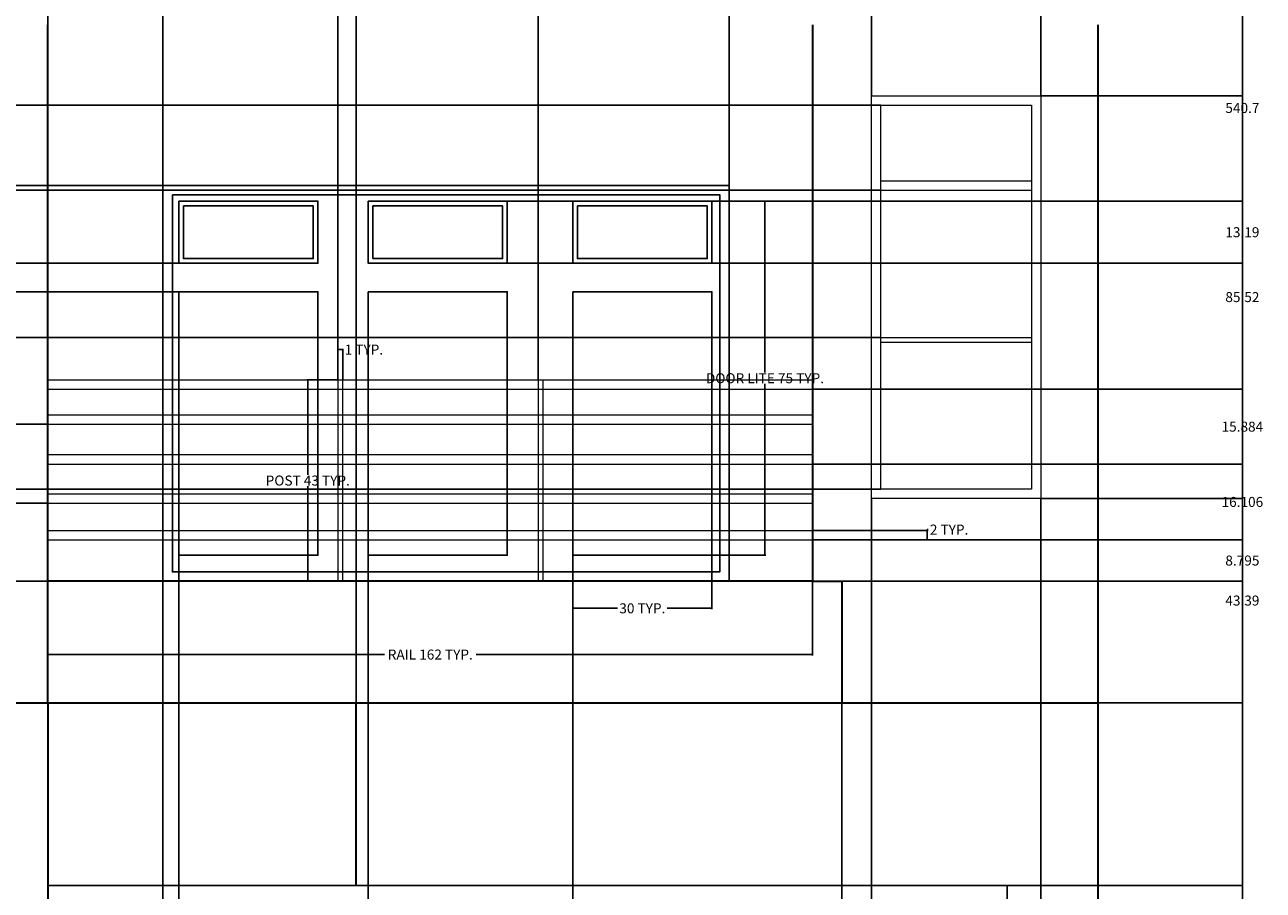
# Model space of a CAD drawing. Units: inches. Extents: x -113 to 379, y 13 to 689.
# Tile 3 of 5: x 116 to 379, y 221 to 405. Entities that reach past the tile are written whole.
import ezdxf

# ---------------------------------------------------------------- set-up
doc = ezdxf.new("R2010")
doc.units = ezdxf.units.IN
doc.header["$MEASUREMENT"] = 0
for name, color, linetype, lineweight in [('A-ANNO-DIMS', 2, 'Continuous', 18), ('A-DOOR', 3, 'Continuous', 25), ('A-FLOR', 7, 'Continuous', 30), ('A-FLOR-HRAL', 5, 'Continuous', 18), ('A-GLAZ', 4, 'Continuous', 18), ('A-WALL', 7, 'Continuous', 35)]:
    doc.layers.add(name, color=color, linetype=linetype, lineweight=lineweight)
doc.styles.get("Standard").update_dxf_attribs({"font": 'arial.ttf'})
doc.dimstyles.get("Standard").update_dxf_attribs({"dimtxt": 2.125, "dimasz": 0.18, "dimexe": 0.18, "dimexo": 0.0625, "dimgap": 0.09, "dimtad": 0, "dimtih": 1, "dimtoh": 1, "dimdec": 4, "dimzin": 0, "dimdsep": 46, "dimlunit": 4, "dimtxsty": 'Standard', "dimcen": 0.09, "dimadec": 0, "dimazin": 0, "dimtfac": 1, "dimtdec": 4, "dimtofl": 0, "dimtmove": 0, "dimatfit": 3, "dimfxl": 1, "dimtolj": 1, "dimtzin": 0, "dimarcsym": 0})

# ---------------------------------------------------------------- blocks, each defined once
blk = doc.blocks.new('BALCONY-DOOR-LITE')
for points in [[(0, 75.21), (29.55, 75.21), (29.55, 62.02), (0, 62.02)], [(1, 74.21), (28.55, 74.21), (28.55, 63.02), (1, 63.02)], [(0, 55.96), (29.55, 55.96), (29.55, 0), (0, 0)]]:
    blk.add_lwpolyline(points, close=True)
blk = doc.blocks.new('BALCONY-RAIL')
for p, q in [((0, 2), (162.45, 2)), ((0, 0), (162.45, 0))]:
    blk.add_line(p, q)
blk = doc.blocks.new('BALCONY-RAIL-POST')
for p, q in [((0, 42.78), (0, 0)), ((1, 42.78), (1, 0))]:
    blk.add_line(p, q)
blk = doc.blocks.new('*D13')
at = {"layer": 'A-ANNO-DIMS', "color": 0, "lineweight": -2, "transparency": 16777216}
for p, q in [((261.87, 367.18), (273.26, 367.18)), ((273.08, 367), (273.08, 330.77)), ((273.08, 292.16), (273.08, 328.39)), ((261.87, 291.98), (273.26, 291.98))]:
    blk.add_line(p, q, dxfattribs=at)
at = {"layer": 'A-ANNO-DIMS', "color": 0, "transparency": 16777216}
for points in [[(273.05, 367), (273.11, 367), (273.08, 367.18)], [(273.05, 292.16), (273.11, 292.16), (273.08, 291.98)]]:
    blk.add_solid(points, dxfattribs=at)
at = {"layer": 'Defpoints', "color": 0, "transparency": 16777216}
for p in [(261.8, 367.18), (273.08, 367.18), (261.8, 291.98)]:
    blk.add_point(p, dxfattribs=at)
at = {"layer": 'A-ANNO-DIMS', "color": 0, "transparency": 16777216, "insert": (273.08, 329.58), "char_height": 2.125, "attachment_point": 5}
blk.add_mtext('\\A1;DOOR LITE 75 TYP.', dxfattribs=at)
blk = doc.blocks.new('*D14')
at = {"layer": 'A-ANNO-DIMS', "color": 0, "lineweight": -2, "transparency": 16777216}
for p, q in [((232.25, 291.91), (232.25, 280.52)), ((261.8, 291.91), (261.8, 280.52)), ((232.43, 280.7), (241.77, 280.7)), ((261.62, 280.7), (252.29, 280.7))]:
    blk.add_line(p, q, dxfattribs=at)
at = {"layer": 'A-ANNO-DIMS', "color": 0, "transparency": 16777216}
for points in [[(232.43, 280.73), (232.43, 280.67), (232.25, 280.7)], [(261.62, 280.73), (261.62, 280.67), (261.8, 280.7)]]:
    blk.add_solid(points, dxfattribs=at)
at = {"layer": 'Defpoints', "color": 0, "transparency": 16777216}
for p in [(232.25, 291.98), (261.8, 291.98), (261.8, 280.7)]:
    blk.add_point(p, dxfattribs=at)
at = {"layer": 'A-ANNO-DIMS', "color": 0, "transparency": 16777216, "insert": (247.03, 280.7), "char_height": 2.125, "attachment_point": 5}
blk.add_mtext('\\A1;30 TYP.', dxfattribs=at)
blk = doc.blocks.new('*D15')
at = {"layer": 'A-ANNO-DIMS', "color": 0, "lineweight": -2, "transparency": 16777216}
for p, q in [((120.75, 295.18), (120.75, 270.7)), ((283.2, 295.18), (283.2, 270.7)), ((120.93, 270.88), (192.23, 270.88)), ((283.02, 270.88), (211.72, 270.88))]:
    blk.add_line(p, q, dxfattribs=at)
at = {"layer": 'A-ANNO-DIMS', "color": 0, "transparency": 16777216}
for points in [[(120.93, 270.91), (120.93, 270.85), (120.75, 270.88)], [(283.02, 270.91), (283.02, 270.85), (283.2, 270.88)]]:
    blk.add_solid(points, dxfattribs=at)
at = {"layer": 'Defpoints', "color": 0, "transparency": 16777216}
for p in [(120.75, 295.24), (283.2, 295.24), (283.2, 270.88)]:
    blk.add_point(p, dxfattribs=at)
at = {"layer": 'A-ANNO-DIMS', "color": 0, "transparency": 16777216, "insert": (201.98, 270.88), "char_height": 2.125, "attachment_point": 5}
blk.add_mtext('\\A1;RAIL 162 TYP.', dxfattribs=at)
blk = doc.blocks.new('*D16')
at = {"layer": 'A-ANNO-DIMS', "color": 0, "lineweight": -2, "transparency": 16777216}
for p, q in [((307.57, 297.24), (307.57, 297.42)), ((307.57, 297.42), (307.75, 297.42)), ((283.26, 297.24), (307.75, 297.24)), ((283.26, 295.24), (307.75, 295.24)), ((307.57, 295.42), (307.57, 297.06))]:
    blk.add_line(p, q, dxfattribs=at)
at = {"layer": 'A-ANNO-DIMS', "color": 0, "transparency": 16777216}
for points in [[(307.54, 297.06), (307.6, 297.06), (307.57, 297.24)], [(307.54, 295.42), (307.6, 295.42), (307.57, 295.24)]]:
    blk.add_solid(points, dxfattribs=at)
at = {"layer": 'Defpoints', "color": 0, "transparency": 16777216}
for p in [(283.2, 297.24), (283.2, 295.24), (307.57, 297.24)]:
    blk.add_point(p, dxfattribs=at)
at = {"layer": 'A-ANNO-DIMS', "color": 0, "transparency": 16777216, "insert": (312.2, 297.42), "char_height": 2.125, "attachment_point": 5}
blk.add_mtext('\\A1;2 TYP.', dxfattribs=at)
blk = doc.blocks.new('*D17')
at = {"layer": 'A-ANNO-DIMS', "color": 0, "lineweight": -2, "transparency": 16777216}
for p, q in [((182.31, 329.23), (175.77, 329.23)), ((175.95, 329.05), (175.95, 309.03)), ((175.95, 286.63), (175.95, 306.65)), ((182.31, 286.45), (175.77, 286.45))]:
    blk.add_line(p, q, dxfattribs=at)
at = {"layer": 'A-ANNO-DIMS', "color": 0, "transparency": 16777216}
for points in [[(175.92, 329.05), (175.98, 329.05), (175.95, 329.23)], [(175.92, 286.63), (175.98, 286.63), (175.95, 286.45)]]:
    blk.add_solid(points, dxfattribs=at)
at = {"layer": 'Defpoints', "color": 0, "transparency": 16777216}
for p in [(175.95, 329.23), (182.37, 329.23), (182.37, 286.45)]:
    blk.add_point(p, dxfattribs=at)
at = {"layer": 'A-ANNO-DIMS', "color": 0, "transparency": 16777216, "insert": (175.95, 307.84), "char_height": 2.125, "attachment_point": 5}
blk.add_mtext('\\A1;POST 43 TYP.', dxfattribs=at)
blk = doc.blocks.new('*D18')
at = {"layer": 'A-ANNO-DIMS', "color": 0, "lineweight": -2, "transparency": 16777216}
for p, q in [((182.37, 329.3), (182.37, 335.83)), ((182.55, 335.65), (183.19, 335.65)), ((183.37, 329.3), (183.37, 335.83)), ((183.37, 335.65), (183.55, 335.65))]:
    blk.add_line(p, q, dxfattribs=at)
at = {"layer": 'A-ANNO-DIMS', "color": 0, "transparency": 16777216}
for points in [[(182.55, 335.68), (182.55, 335.62), (182.37, 335.65)], [(183.19, 335.68), (183.19, 335.62), (183.37, 335.65)]]:
    blk.add_solid(points, dxfattribs=at)
at = {"layer": 'Defpoints', "color": 0, "transparency": 16777216}
for p in [(183.37, 335.65), (182.37, 329.23), (183.37, 329.23)]:
    blk.add_point(p, dxfattribs=at)
at = {"layer": 'A-ANNO-DIMS', "color": 0, "transparency": 16777216, "insert": (187.88, 335.65), "char_height": 2.125, "attachment_point": 5}
blk.add_mtext('\\A1;1 TYP.', dxfattribs=at)
blk = doc.blocks.new('*D20')
at = {"layer": 'A-ANNO-DIMS', "color": 0, "lineweight": -2, "transparency": 16777216}
for p, q in [((232.74, 657.3), (374.68, 657.3)), ((374.5, 657.12), (374.5, 388.15)), ((374.5, 116.83), (374.5, 385.8)), ((343.93, 116.65), (374.68, 116.65))]:
    blk.add_line(p, q, dxfattribs=at)
at = {"layer": 'A-ANNO-DIMS', "color": 0, "transparency": 16777216}
for points in [[(374.47, 657.12), (374.53, 657.12), (374.5, 657.3)], [(374.47, 116.83), (374.53, 116.83), (374.5, 116.65)]]:
    blk.add_solid(points, dxfattribs=at)
at = {"layer": 'Defpoints', "color": 0, "transparency": 16777216}
for p in [(232.68, 657.3), (374.5, 657.3), (343.87, 116.65)]:
    blk.add_point(p, dxfattribs=at)
at = {"layer": 'A-ANNO-DIMS', "color": 0, "transparency": 16777216, "insert": (374.5, 386.98), "char_height": 2.125, "attachment_point": 5}
blk.add_mtext('\\A1;540.7', dxfattribs=at)
blk = doc.blocks.new('*D33')
at = {"layer": 'A-ANNO-DIMS', "color": 0, "lineweight": -2, "transparency": 16777216}
for p, q in [((120.75, 221.89), (120.75, 688.12)), ((120.93, 687.94), (149.81, 687.94)), ((186.04, 687.94), (157.17, 687.94)), ((186.22, 221.89), (186.22, 688.12))]:
    blk.add_line(p, q, dxfattribs=at)
at = {"layer": 'A-ANNO-DIMS', "color": 0, "transparency": 16777216}
for points in [[(120.93, 687.97), (120.93, 687.91), (120.75, 687.94)], [(186.04, 687.97), (186.04, 687.91), (186.22, 687.94)]]:
    blk.add_solid(points, dxfattribs=at)
at = {"layer": 'Defpoints', "color": 0, "transparency": 16777216}
for p in [(186.22, 687.94), (120.75, 221.82), (186.22, 221.82)]:
    blk.add_point(p, dxfattribs=at)
at = {"layer": 'A-ANNO-DIMS', "color": 0, "transparency": 16777216, "insert": (153.49, 687.94), "char_height": 2.125, "attachment_point": 5}
blk.add_mtext('\\A1;65.47', dxfattribs=at)
blk = doc.blocks.new('*D35')
at = {"layer": 'A-ANNO-DIMS', "color": 0, "lineweight": -2, "transparency": 16777216}
for p, q in [((324.57, 221.82), (374.68, 221.82)), ((374.5, 221.64), (374.5, 170.41)), ((374.5, 116.83), (374.5, 168.06)), ((324.57, 116.65), (374.68, 116.65))]:
    blk.add_line(p, q, dxfattribs=at)
at = {"layer": 'A-ANNO-DIMS', "color": 0, "transparency": 16777216}
for points in [[(374.47, 221.64), (374.53, 221.64), (374.5, 221.82)], [(374.47, 116.83), (374.53, 116.83), (374.5, 116.65)]]:
    blk.add_solid(points, dxfattribs=at)
at = {"layer": 'Defpoints', "color": 0, "transparency": 16777216}
for p in [(324.51, 221.82), (374.5, 221.82), (324.51, 116.65)]:
    blk.add_point(p, dxfattribs=at)
at = {"layer": 'A-ANNO-DIMS', "color": 0, "transparency": 16777216, "insert": (374.5, 169.24), "char_height": 2.125, "attachment_point": 5}
blk.add_mtext('\\A1;105.17', dxfattribs=at)
blk = doc.blocks.new('*D38')
at = {"layer": 'A-ANNO-DIMS', "color": 0, "lineweight": -2, "transparency": 16777216}
for p, q in [((289.33, 286.45), (-108.66, 286.45)), ((-108.48, 286.27), (-108.48, 274.73)), ((-108.48, 260.83), (-108.48, 272.38)), ((289.33, 260.65), (-108.66, 260.65))]:
    blk.add_line(p, q, dxfattribs=at)
at = {"layer": 'A-ANNO-DIMS', "color": 0, "transparency": 16777216}
for points in [[(-108.51, 286.27), (-108.45, 286.27), (-108.48, 286.45)], [(-108.51, 260.83), (-108.45, 260.83), (-108.48, 260.65)]]:
    blk.add_solid(points, dxfattribs=at)
at = {"layer": 'Defpoints', "color": 0, "transparency": 16777216}
for p in [(-108.48, 286.45), (289.4, 286.45), (289.4, 260.65)]:
    blk.add_point(p, dxfattribs=at)
at = {"layer": 'A-ANNO-DIMS', "color": 0, "transparency": 16777216, "insert": (-108.48, 273.55), "char_height": 2.125, "attachment_point": 5}
blk.add_mtext('\\A1;25.8', dxfattribs=at)
blk = doc.blocks.new('*D39')
at = {"layer": 'A-ANNO-DIMS', "color": 0, "lineweight": -2, "transparency": 16777216}
for p, q in [((145.2, 370.61), (145.2, 688.12)), ((145.38, 687.94), (201.77, 687.94)), ((265.31, 687.94), (208.92, 687.94)), ((265.49, 370.61), (265.49, 688.12))]:
    blk.add_line(p, q, dxfattribs=at)
at = {"layer": 'A-ANNO-DIMS', "color": 0, "transparency": 16777216}
for points in [[(145.38, 687.97), (145.38, 687.91), (145.2, 687.94)], [(265.31, 687.97), (265.31, 687.91), (265.49, 687.94)]]:
    blk.add_solid(points, dxfattribs=at)
at = {"layer": 'Defpoints', "color": 0, "transparency": 16777216}
for p in [(265.49, 687.94), (145.2, 370.54), (265.49, 370.54)]:
    blk.add_point(p, dxfattribs=at)
at = {"layer": 'A-ANNO-DIMS', "color": 0, "transparency": 16777216, "insert": (205.34, 687.94), "char_height": 2.125, "attachment_point": 5}
blk.add_mtext('\\A1;120.3', dxfattribs=at)
blk = doc.blocks.new('*D40')
at = {"layer": 'A-ANNO-DIMS', "color": 0, "lineweight": -2, "transparency": 16777216}
for p, q in [((145.14, 370.54), (-108.66, 370.54)), ((-108.48, 370.36), (-108.48, 329.67)), ((-108.48, 286.63), (-108.48, 327.32)), ((145.14, 286.45), (-108.66, 286.45))]:
    blk.add_line(p, q, dxfattribs=at)
at = {"layer": 'A-ANNO-DIMS', "color": 0, "transparency": 16777216}
for points in [[(-108.51, 370.36), (-108.45, 370.36), (-108.48, 370.54)], [(-108.51, 286.63), (-108.45, 286.63), (-108.48, 286.45)]]:
    blk.add_solid(points, dxfattribs=at)
at = {"layer": 'Defpoints', "color": 0, "transparency": 16777216}
for p in [(-108.48, 370.54), (145.2, 370.54), (145.2, 286.45)]:
    blk.add_point(p, dxfattribs=at)
at = {"layer": 'A-ANNO-DIMS', "color": 0, "transparency": 16777216, "insert": (-108.48, 328.5), "char_height": 2.125, "attachment_point": 5}
blk.add_mtext('\\A1;84.1', dxfattribs=at)
blk = doc.blocks.new('*D41')
at = {"layer": 'A-ANNO-DIMS', "color": 0, "lineweight": -2, "transparency": 16777216}
for p, q in [((120.75, 286.39), (120.75, 13.95)), ((145.2, 286.39), (145.2, 13.95)), ((120.93, 14.13), (128.45, 14.13)), ((145.02, 14.13), (137.5, 14.13))]:
    blk.add_line(p, q, dxfattribs=at)
at = {"layer": 'A-ANNO-DIMS', "color": 0, "transparency": 16777216}
for points in [[(120.93, 14.16), (120.93, 14.1), (120.75, 14.13)], [(145.02, 14.16), (145.02, 14.1), (145.2, 14.13)]]:
    blk.add_solid(points, dxfattribs=at)
at = {"layer": 'Defpoints', "color": 0, "transparency": 16777216}
for p in [(120.75, 286.45), (145.2, 286.45), (145.2, 14.13)]:
    blk.add_point(p, dxfattribs=at)
at = {"layer": 'A-ANNO-DIMS', "color": 0, "transparency": 16777216, "insert": (132.98, 14.13), "char_height": 2.125, "attachment_point": 5}
blk.add_mtext('\\A1;24.445', dxfattribs=at)
blk = doc.blocks.new('*D42')
at = {"layer": 'A-ANNO-DIMS', "color": 0, "lineweight": -2, "transparency": 16777216}
for p, q in [((295.73, 389.63), (295.73, 688.12)), ((295.91, 687.94), (309.2, 687.94)), ((331.5, 687.94), (318.21, 687.94)), ((331.68, 389.63), (331.68, 688.12))]:
    blk.add_line(p, q, dxfattribs=at)
at = {"layer": 'A-ANNO-DIMS', "color": 0, "transparency": 16777216}
for points in [[(295.91, 687.97), (295.91, 687.91), (295.73, 687.94)], [(331.5, 687.97), (331.5, 687.91), (331.68, 687.94)]]:
    blk.add_solid(points, dxfattribs=at)
at = {"layer": 'Defpoints', "color": 0, "transparency": 16777216}
for p in [(331.68, 687.94), (295.73, 389.57), (331.68, 389.57)]:
    blk.add_point(p, dxfattribs=at)
at = {"layer": 'A-ANNO-DIMS', "color": 0, "transparency": 16777216, "insert": (313.71, 687.94), "char_height": 2.125, "attachment_point": 5}
blk.add_mtext('\\A1;35.955', dxfattribs=at)
blk = doc.blocks.new('*D43')
at = {"layer": 'A-ANNO-DIMS', "color": 0, "lineweight": -2, "transparency": 16777216}
for p, q in [((331.75, 389.57), (374.68, 389.57)), ((374.5, 389.39), (374.5, 347.98)), ((374.5, 304.22), (374.5, 345.63)), ((331.75, 304.04), (374.68, 304.04))]:
    blk.add_line(p, q, dxfattribs=at)
at = {"layer": 'A-ANNO-DIMS', "color": 0, "transparency": 16777216}
for points in [[(374.47, 389.39), (374.53, 389.39), (374.5, 389.57)], [(374.47, 304.22), (374.53, 304.22), (374.5, 304.04)]]:
    blk.add_solid(points, dxfattribs=at)
at = {"layer": 'Defpoints', "color": 0, "transparency": 16777216}
for p in [(331.68, 389.57), (374.5, 389.57), (331.68, 304.04)]:
    blk.add_point(p, dxfattribs=at)
at = {"layer": 'A-ANNO-DIMS', "color": 0, "transparency": 16777216, "insert": (374.5, 346.81), "char_height": 2.125, "attachment_point": 5}
blk.add_mtext('\\A1;85.52', dxfattribs=at)
blk = doc.blocks.new('*D44')
at = {"layer": 'A-ANNO-DIMS', "color": 0, "lineweight": -2, "transparency": 16777216}
for p, q in [((331.68, 303.98), (331.68, 13.95)), ((343.87, 260.59), (343.87, 13.95)), ((331.86, 14.13), (333.38, 14.13)), ((343.69, 14.13), (342.18, 14.13))]:
    blk.add_line(p, q, dxfattribs=at)
at = {"layer": 'A-ANNO-DIMS', "color": 0, "transparency": 16777216}
for points in [[(331.86, 14.16), (331.86, 14.1), (331.68, 14.13)], [(343.69, 14.16), (343.69, 14.1), (343.87, 14.13)]]:
    blk.add_solid(points, dxfattribs=at)
at = {"layer": 'Defpoints', "color": 0, "transparency": 16777216}
for p in [(331.68, 304.04), (343.87, 260.65), (343.87, 14.13)]:
    blk.add_point(p, dxfattribs=at)
at = {"layer": 'A-ANNO-DIMS', "color": 0, "transparency": 16777216, "insert": (337.78, 14.13), "char_height": 2.125, "attachment_point": 5}
blk.add_mtext('\\A1;12.186', dxfattribs=at)
blk = doc.blocks.new('*D45')
at = {"layer": 'A-ANNO-DIMS', "color": 0, "lineweight": -2, "transparency": 16777216}
for p, q in [((331.75, 304.04), (374.68, 304.04)), ((374.5, 303.86), (374.5, 283.52)), ((374.5, 260.83), (374.5, 281.17)), ((343.93, 260.65), (374.68, 260.65))]:
    blk.add_line(p, q, dxfattribs=at)
at = {"layer": 'A-ANNO-DIMS', "color": 0, "transparency": 16777216}
for points in [[(374.47, 303.86), (374.53, 303.86), (374.5, 304.04)], [(374.47, 260.83), (374.53, 260.83), (374.5, 260.65)]]:
    blk.add_solid(points, dxfattribs=at)
at = {"layer": 'Defpoints', "color": 0, "transparency": 16777216}
for p in [(331.68, 304.04), (343.87, 260.65), (374.5, 260.65)]:
    blk.add_point(p, dxfattribs=at)
at = {"layer": 'A-ANNO-DIMS', "color": 0, "transparency": 16777216, "insert": (374.5, 282.35), "char_height": 2.125, "attachment_point": 5}
blk.add_mtext('\\A1;43.39', dxfattribs=at)
blk = doc.blocks.new('*D46')
at = {"layer": 'A-ANNO-DIMS', "color": 0, "lineweight": -2, "transparency": 16777216}
for p, q in [((295.73, 303.98), (295.73, 13.95)), ((289.4, 260.59), (289.4, 13.95)), ((289.58, 14.13), (295.55, 14.13)), ((295.73, 14.13), (295.91, 14.13))]:
    blk.add_line(p, q, dxfattribs=at)
at = {"layer": 'A-ANNO-DIMS', "color": 0, "transparency": 16777216}
for points in [[(289.58, 14.16), (289.58, 14.1), (289.4, 14.13)], [(295.55, 14.16), (295.55, 14.1), (295.73, 14.13)]]:
    blk.add_solid(points, dxfattribs=at)
at = {"layer": 'Defpoints', "color": 0, "transparency": 16777216}
for p in [(295.73, 304.04), (289.4, 260.65), (295.73, 14.13)]:
    blk.add_point(p, dxfattribs=at)
at = {"layer": 'A-ANNO-DIMS', "color": 0, "transparency": 16777216, "insert": (299.58, 14.13), "char_height": 2.125, "attachment_point": 5}
blk.add_mtext('\\A1;6.332', dxfattribs=at)
blk = doc.blocks.new('*D56')
at = {"layer": 'A-ANNO-DIMS', "color": 0, "lineweight": -2, "transparency": 16777216}
for p, q in [((148.55, 291.91), (148.55, 13.95)), ((188.79, 291.91), (188.79, 13.95)), ((148.73, 14.13), (164.96, 14.13)), ((188.61, 14.13), (172.39, 14.13))]:
    blk.add_line(p, q, dxfattribs=at)
at = {"layer": 'A-ANNO-DIMS', "color": 0, "transparency": 16777216}
for points in [[(148.73, 14.16), (148.73, 14.1), (148.55, 14.13)], [(188.61, 14.16), (188.61, 14.1), (188.79, 14.13)]]:
    blk.add_solid(points, dxfattribs=at)
at = {"layer": 'Defpoints', "color": 0, "transparency": 16777216}
for p in [(148.55, 291.98), (188.79, 291.98), (188.79, 14.13)]:
    blk.add_point(p, dxfattribs=at)
at = {"layer": 'A-ANNO-DIMS', "color": 0, "transparency": 16777216, "insert": (168.67, 14.13), "char_height": 2.125, "attachment_point": 5}
blk.add_mtext('\\A1;40.24', dxfattribs=at)
blk = doc.blocks.new('*D57')
at = {"layer": 'A-ANNO-DIMS', "color": 0, "lineweight": -2, "transparency": 16777216}
for p, q in [((188.79, 291.91), (188.79, 13.95)), ((232.25, 291.91), (232.25, 13.95)), ((188.97, 14.13), (206.81, 14.13)), ((232.07, 14.13), (214.24, 14.13))]:
    blk.add_line(p, q, dxfattribs=at)
at = {"layer": 'A-ANNO-DIMS', "color": 0, "transparency": 16777216}
for points in [[(188.97, 14.16), (188.97, 14.1), (188.79, 14.13)], [(232.07, 14.16), (232.07, 14.1), (232.25, 14.13)]]:
    blk.add_solid(points, dxfattribs=at)
at = {"layer": 'Defpoints', "color": 0, "transparency": 16777216}
for p in [(188.79, 291.98), (232.25, 291.98), (232.25, 14.13)]:
    blk.add_point(p, dxfattribs=at)
at = {"layer": 'A-ANNO-DIMS', "color": 0, "transparency": 16777216, "insert": (210.52, 14.13), "char_height": 2.125, "attachment_point": 5}
blk.add_mtext('\\A1;43.46', dxfattribs=at)
blk = doc.blocks.new('*D58')
at = {"layer": 'A-ANNO-DIMS', "color": 0, "lineweight": -2, "transparency": 16777216}
for p, q in [((182.37, 329.3), (182.37, 688.12)), ((182.55, 687.94), (199.91, 687.94)), ((224.72, 687.94), (207.35, 687.94)), ((224.9, 329.3), (224.9, 688.12))]:
    blk.add_line(p, q, dxfattribs=at)
at = {"layer": 'A-ANNO-DIMS', "color": 0, "transparency": 16777216}
for points in [[(182.55, 687.97), (182.55, 687.91), (182.37, 687.94)], [(224.72, 687.97), (224.72, 687.91), (224.9, 687.94)]]:
    blk.add_solid(points, dxfattribs=at)
at = {"layer": 'Defpoints', "color": 0, "transparency": 16777216}
for p in [(224.9, 687.94), (182.37, 329.23), (224.9, 329.23)]:
    blk.add_point(p, dxfattribs=at)
at = {"layer": 'A-ANNO-DIMS', "color": 0, "transparency": 16777216, "insert": (203.63, 687.94), "char_height": 2.125, "attachment_point": 5}
blk.add_mtext('\\A1;42.53', dxfattribs=at)
blk = doc.blocks.new('*D59')
at = {"layer": 'A-ANNO-DIMS', "color": 0, "lineweight": -2, "transparency": 16777216}
for p, q in [((120.75, 329.3), (120.75, 688.12)), ((120.93, 687.94), (148.08, 687.94)), ((182.19, 687.94), (155.04, 687.94)), ((182.37, 329.3), (182.37, 688.12))]:
    blk.add_line(p, q, dxfattribs=at)
at = {"layer": 'A-ANNO-DIMS', "color": 0, "transparency": 16777216}
for points in [[(120.93, 687.97), (120.93, 687.91), (120.75, 687.94)], [(182.19, 687.97), (182.19, 687.91), (182.37, 687.94)]]:
    blk.add_solid(points, dxfattribs=at)
at = {"layer": 'Defpoints', "color": 0, "transparency": 16777216}
for p in [(182.37, 687.94), (120.75, 329.23), (182.37, 329.23)]:
    blk.add_point(p, dxfattribs=at)
at = {"layer": 'A-ANNO-DIMS', "color": 0, "transparency": 16777216, "insert": (151.56, 687.94), "char_height": 2.125, "attachment_point": 5}
blk.add_mtext('\\A1;61.61', dxfattribs=at)
blk = doc.blocks.new('*D60')
at = {"layer": 'A-ANNO-DIMS', "color": 0, "lineweight": -2, "transparency": 16777216}
for p, q in [((120.69, 303.02), (-108.66, 303.02)), ((-108.48, 302.84), (-108.48, 295.91)), ((-108.48, 286.63), (-108.48, 293.56)), ((120.69, 286.45), (-108.66, 286.45))]:
    blk.add_line(p, q, dxfattribs=at)
at = {"layer": 'A-ANNO-DIMS', "color": 0, "transparency": 16777216}
for points in [[(-108.51, 302.84), (-108.45, 302.84), (-108.48, 303.02)], [(-108.51, 286.63), (-108.45, 286.63), (-108.48, 286.45)]]:
    blk.add_solid(points, dxfattribs=at)
at = {"layer": 'Defpoints', "color": 0, "transparency": 16777216}
for p in [(-108.48, 303.02), (120.75, 303.02), (120.75, 286.45)]:
    blk.add_point(p, dxfattribs=at)
at = {"layer": 'A-ANNO-DIMS', "color": 0, "transparency": 16777216, "insert": (-108.48, 294.73), "char_height": 2.125, "attachment_point": 5}
blk.add_mtext('\\A1;16.566', dxfattribs=at)
blk = doc.blocks.new('*D61')
at = {"layer": 'A-ANNO-DIMS', "color": 0, "lineweight": -2, "transparency": 16777216}
for p, q in [((120.69, 319.8), (-108.66, 319.8)), ((-108.48, 319.62), (-108.48, 312.58)), ((-108.48, 303.2), (-108.48, 310.23)), ((120.69, 303.02), (-108.66, 303.02))]:
    blk.add_line(p, q, dxfattribs=at)
at = {"layer": 'A-ANNO-DIMS', "color": 0, "transparency": 16777216}
for points in [[(-108.51, 319.62), (-108.45, 319.62), (-108.48, 319.8)], [(-108.51, 303.2), (-108.45, 303.2), (-108.48, 303.02)]]:
    blk.add_solid(points, dxfattribs=at)
at = {"layer": 'Defpoints', "color": 0, "transparency": 16777216}
for p in [(-108.48, 319.8), (120.75, 319.8), (120.75, 303.02)]:
    blk.add_point(p, dxfattribs=at)
at = {"layer": 'A-ANNO-DIMS', "color": 0, "transparency": 16777216, "insert": (-108.48, 311.41), "char_height": 2.125, "attachment_point": 5}
blk.add_mtext('\\A1;16.788', dxfattribs=at)
blk = doc.blocks.new('*D62')
at = {"layer": 'A-ANNO-DIMS', "color": 0, "lineweight": -2, "transparency": 16777216}
for p, q in [((283.26, 295.24), (374.68, 295.24)), ((374.5, 295.06), (374.5, 292.02)), ((374.5, 286.63), (374.5, 289.67)), ((283.26, 286.45), (374.68, 286.45))]:
    blk.add_line(p, q, dxfattribs=at)
at = {"layer": 'A-ANNO-DIMS', "color": 0, "transparency": 16777216}
for points in [[(374.47, 295.06), (374.53, 295.06), (374.5, 295.24)], [(374.47, 286.63), (374.53, 286.63), (374.5, 286.45)]]:
    blk.add_solid(points, dxfattribs=at)
at = {"layer": 'Defpoints', "color": 0, "transparency": 16777216}
for p in [(283.2, 295.24), (374.5, 295.24), (283.2, 286.45)]:
    blk.add_point(p, dxfattribs=at)
at = {"layer": 'A-ANNO-DIMS', "color": 0, "transparency": 16777216, "insert": (374.5, 290.85), "char_height": 2.125, "attachment_point": 5}
blk.add_mtext('\\A1;8.795', dxfattribs=at)
blk = doc.blocks.new('*D63')
at = {"layer": 'A-ANNO-DIMS', "color": 0, "lineweight": -2, "transparency": 16777216}
for p, q in [((283.26, 311.35), (374.68, 311.35)), ((374.5, 311.17), (374.5, 304.47)), ((374.5, 295.42), (374.5, 302.12)), ((283.26, 295.24), (374.68, 295.24))]:
    blk.add_line(p, q, dxfattribs=at)
at = {"layer": 'A-ANNO-DIMS', "color": 0, "transparency": 16777216}
for points in [[(374.47, 311.17), (374.53, 311.17), (374.5, 311.35)], [(374.47, 295.42), (374.53, 295.42), (374.5, 295.24)]]:
    blk.add_solid(points, dxfattribs=at)
at = {"layer": 'Defpoints', "color": 0, "transparency": 16777216}
for p in [(283.2, 311.35), (374.5, 311.35), (283.2, 295.24)]:
    blk.add_point(p, dxfattribs=at)
at = {"layer": 'A-ANNO-DIMS', "color": 0, "transparency": 16777216, "insert": (374.5, 303.3), "char_height": 2.125, "attachment_point": 5}
blk.add_mtext('\\A1;16.106', dxfattribs=at)
blk = doc.blocks.new('*D64')
at = {"layer": 'A-ANNO-DIMS', "color": 0, "lineweight": -2, "transparency": 16777216}
for p, q in [((283.26, 327.23), (374.68, 327.23)), ((374.5, 327.05), (374.5, 320.47)), ((374.5, 311.53), (374.5, 318.12)), ((283.26, 311.35), (374.68, 311.35))]:
    blk.add_line(p, q, dxfattribs=at)
at = {"layer": 'A-ANNO-DIMS', "color": 0, "transparency": 16777216}
for points in [[(374.47, 327.05), (374.53, 327.05), (374.5, 327.23)], [(374.47, 311.53), (374.53, 311.53), (374.5, 311.35)]]:
    blk.add_solid(points, dxfattribs=at)
at = {"layer": 'Defpoints', "color": 0, "transparency": 16777216}
for p in [(283.2, 327.23), (374.5, 327.23), (283.2, 311.35)]:
    blk.add_point(p, dxfattribs=at)
at = {"layer": 'A-ANNO-DIMS', "color": 0, "transparency": 16777216, "insert": (374.5, 319.29), "char_height": 2.125, "attachment_point": 5}
blk.add_mtext('\\A1;15.884', dxfattribs=at)
blk = doc.blocks.new('*D65')
at = {"layer": 'A-ANNO-DIMS', "color": 0, "lineweight": -2, "transparency": 16777216}
for p, q in [((297.67, 338.26), (-108.66, 338.26)), ((-108.48, 338.08), (-108.48, 323.33)), ((-108.48, 306.22), (-108.48, 320.98)), ((297.67, 306.04), (-108.66, 306.04))]:
    blk.add_line(p, q, dxfattribs=at)
at = {"layer": 'A-ANNO-DIMS', "color": 0, "transparency": 16777216}
for points in [[(-108.51, 338.08), (-108.45, 338.08), (-108.48, 338.26)], [(-108.51, 306.22), (-108.45, 306.22), (-108.48, 306.04)]]:
    blk.add_solid(points, dxfattribs=at)
at = {"layer": 'Defpoints', "color": 0, "transparency": 16777216}
for p in [(-108.48, 338.26), (297.73, 338.26), (297.73, 306.04)]:
    blk.add_point(p, dxfattribs=at)
at = {"layer": 'A-ANNO-DIMS', "color": 0, "transparency": 16777216, "insert": (-108.48, 322.15), "char_height": 2.125, "attachment_point": 5}
blk.add_mtext('\\A1;32.21', dxfattribs=at)
blk = doc.blocks.new('*D66')
at = {"layer": 'A-ANNO-DIMS', "color": 0, "lineweight": -2, "transparency": 16777216}
for p, q in [((297.67, 369.51), (-108.66, 369.51)), ((-108.48, 369.33), (-108.48, 355.06)), ((-108.48, 338.44), (-108.48, 352.71)), ((297.67, 338.26), (-108.66, 338.26))]:
    blk.add_line(p, q, dxfattribs=at)
at = {"layer": 'A-ANNO-DIMS', "color": 0, "transparency": 16777216}
for points in [[(-108.51, 369.33), (-108.45, 369.33), (-108.48, 369.51)], [(-108.51, 338.44), (-108.45, 338.44), (-108.48, 338.26)]]:
    blk.add_solid(points, dxfattribs=at)
at = {"layer": 'Defpoints', "color": 0, "transparency": 16777216}
for p in [(-108.48, 369.51), (297.73, 369.51), (297.73, 338.26)]:
    blk.add_point(p, dxfattribs=at)
at = {"layer": 'A-ANNO-DIMS', "color": 0, "transparency": 16777216, "insert": (-108.48, 353.88), "char_height": 2.125, "attachment_point": 5}
blk.add_mtext('\\A1;31.254', dxfattribs=at)
blk = doc.blocks.new('*D67')
at = {"layer": 'A-ANNO-DIMS', "color": 0, "lineweight": -2, "transparency": 16777216}
for p, q in [((297.67, 387.57), (-108.66, 387.57)), ((-108.48, 387.39), (-108.48, 379.71)), ((-108.48, 369.69), (-108.48, 377.36)), ((297.67, 369.51), (-108.66, 369.51))]:
    blk.add_line(p, q, dxfattribs=at)
at = {"layer": 'A-ANNO-DIMS', "color": 0, "transparency": 16777216}
for points in [[(-108.51, 387.39), (-108.45, 387.39), (-108.48, 387.57)], [(-108.51, 369.69), (-108.45, 369.69), (-108.48, 369.51)]]:
    blk.add_solid(points, dxfattribs=at)
at = {"layer": 'Defpoints', "color": 0, "transparency": 16777216}
for p in [(-108.48, 387.57), (297.73, 387.57), (297.73, 369.51)]:
    blk.add_point(p, dxfattribs=at)
at = {"layer": 'A-ANNO-DIMS', "color": 0, "transparency": 16777216, "insert": (-108.48, 378.54), "char_height": 2.125, "attachment_point": 5}
blk.add_mtext('\\A1;18.056', dxfattribs=at)
blk = doc.blocks.new('*D68')
at = {"layer": 'A-ANNO-DIMS', "color": 0, "lineweight": -2, "transparency": 16777216}
for p, q in [((218.41, 367.18), (374.68, 367.18)), ((374.5, 367), (374.5, 361.76)), ((374.5, 354.17), (374.5, 359.41)), ((218.41, 353.99), (374.68, 353.99))]:
    blk.add_line(p, q, dxfattribs=at)
at = {"layer": 'A-ANNO-DIMS', "color": 0, "transparency": 16777216}
for points in [[(374.47, 367), (374.53, 367), (374.5, 367.18)], [(374.47, 354.17), (374.53, 354.17), (374.5, 353.99)]]:
    blk.add_solid(points, dxfattribs=at)
at = {"layer": 'Defpoints', "color": 0, "transparency": 16777216}
for p in [(218.34, 367.18), (218.34, 353.99), (374.5, 353.99)]:
    blk.add_point(p, dxfattribs=at)
at = {"layer": 'A-ANNO-DIMS', "color": 0, "transparency": 16777216, "insert": (374.5, 360.59), "char_height": 2.125, "attachment_point": 5}
blk.add_mtext('\\A1;13.19', dxfattribs=at)
blk = doc.blocks.new('*D69')
at = {"layer": 'A-ANNO-DIMS', "color": 0, "lineweight": -2, "transparency": 16777216}
for p, q in [((148.49, 353.99), (-108.66, 353.99)), ((-108.48, 353.81), (-108.48, 352.14)), ((148.49, 347.94), (-108.66, 347.94)), ((-108.48, 348.12), (-108.48, 349.79))]:
    blk.add_line(p, q, dxfattribs=at)
at = {"layer": 'A-ANNO-DIMS', "color": 0, "transparency": 16777216}
for points in [[(-108.51, 353.81), (-108.45, 353.81), (-108.48, 353.99)], [(-108.51, 348.12), (-108.45, 348.12), (-108.48, 347.94)]]:
    blk.add_solid(points, dxfattribs=at)
at = {"layer": 'Defpoints', "color": 0, "transparency": 16777216}
for p in [(148.55, 353.99), (-108.48, 347.94), (148.55, 347.94)]:
    blk.add_point(p, dxfattribs=at)
at = {"layer": 'A-ANNO-DIMS', "color": 0, "transparency": 16777216, "insert": (-108.48, 350.97), "char_height": 2.125, "attachment_point": 5}
blk.add_mtext('\\A1;6.056', dxfattribs=at)

msp = doc.modelspace()

# ---------------------------------------------------------------- linework, layer by layer
at = {"layer": 'A-DOOR'}
for points in [[(145.1985, 370.5425), (265.4865, 370.5425), (265.4865, 286.4497), (145.1985, 286.4497)], [(147.1985, 368.5425), (263.4865, 368.5425), (263.4865, 288.4497), (147.1985, 288.4497)], [(120.7533, 221.8228), (324.5073, 221.8228), (324.5073, 116.6509), (120.7533, 116.6509)]]:
    msp.add_lwpolyline(points, close=True, dxfattribs=at)
at = {"layer": 'A-FLOR'}
for p, q in [((283.2008, 286.4497), (120.7533, 286.4497)), ((283.2008, 286.4497), (289.3958, 286.4497)), ((289.3958, 286.4497), (289.3958, 260.6509)), ((81.8721, 260.6509), (129.5137, 260.6509)), ((129.5137, 260.6509), (343.8693, 260.6509))]:
    msp.add_line(p, q, dxfattribs=at)
at = {"layer": 'A-GLAZ'}
for p, q in [((297.728, 371.5111), (329.6831, 371.5111)), ((297.728, 369.5111), (329.6831, 369.5111)), ((297.728, 338.2572), (329.6831, 338.2572)), ((297.728, 337.2572), (329.6831, 337.2572))]:
    msp.add_line(p, q, dxfattribs=at)
for points in [[(295.728, 389.5666), (331.6831, 389.5666), (331.6831, 304.0445), (295.728, 304.0445)], [(297.728, 387.5666), (329.6831, 387.5666), (329.6831, 306.0445), (297.728, 306.0445)]]:
    msp.add_lwpolyline(points, close=True, dxfattribs=at)
at = {"layer": 'A-WALL'}
for p, q in [((120.7533, 260.6509), (120.7533, 404.6509)), ((283.2008, 404.6509), (283.2008, 292.0582)), ((343.8693, 260.6509), (343.8693, 404.6509)), ((283.2008, 292.0582), (283.2008, 286.4497)), ((120.7533, 260.6509), (120.7533, 116.6509)), ((186.2204, 221.8228), (186.2204, 260.6509)), ((343.8693, 116.6509), (343.8693, 260.6509))]:
    msp.add_line(p, q, dxfattribs=at)

# ---------------------------------------------------------------- block references
at = {"layer": 'A-DOOR'}
for p in [(148.5524, 291.9762), (188.7939, 291.9762), (232.2544, 291.9762)]:
    msp.add_blockref('BALCONY-DOOR-LITE', p, dxfattribs=at)
at = {"layer": 'A-FLOR-HRAL'}
for name, p in [('BALCONY-RAIL', (120.7533, 327.234)), ('BALCONY-RAIL-POST', (182.3676, 286.4497)), ('BALCONY-RAIL-POST', (224.8984, 286.4497)), ('BALCONY-RAIL', (120.7533, 319.8035)), ('BALCONY-RAIL', (120.7533, 311.3505)), ('BALCONY-RAIL', (120.7533, 303.016)), ('BALCONY-RAIL', (120.7533, 295.2447))]:
    msp.add_blockref(name, p, dxfattribs=at)

# ---------------------------------------------------------------- dimensions: what is measured, and where the dimension line sits
at = {"layer": 'A-ANNO-DIMS'}
for base, p1, p2, override, picture, middle in [((186.2204, 687.9364), (120.7533, 221.8228), (186.2204, 221.8228), {"dimdec": 2, "dimlfac": 1, "dimrnd": 0, "dimzin": 0, "dimdsep": 46, "dimlunit": 2}, '*D33', (153.4869, 687.9364)), ((182.3676, 687.9364), (120.7533, 329.234), (182.3676, 329.234), {"dimdec": 2, "dimlfac": 1, "dimrnd": 0, "dimzin": 0, "dimdsep": 46, "dimlunit": 2}, '*D59', (151.5604, 687.9364)), ((265.4865, 687.9364), (145.1985, 370.5425), (265.4865, 370.5425), {"dimdec": 1, "dimlfac": 1, "dimrnd": 0, "dimzin": 0, "dimdsep": 46, "dimlunit": 2}, '*D39', (205.3425, 687.9364)), ((224.8984, 687.9364), (182.3676, 329.234), (224.8984, 329.234), {"dimdec": 2, "dimlfac": 1, "dimrnd": 0, "dimzin": 0, "dimdsep": 46, "dimlunit": 2}, '*D58', (203.633, 687.9364)), ((331.6831, 687.9364), (295.728, 389.5666), (331.6831, 389.5666), {"dimdec": 3, "dimlfac": 1, "dimrnd": 0, "dimzin": 0, "dimdsep": 46, "dimlunit": 2}, '*D42', (313.7055, 687.9364)), ((295.728, 14.1289), (289.3958, 260.6509), (295.728, 304.0445), {"dimdec": 3, "dimlfac": 1, "dimrnd": 0, "dimzin": 0, "dimdsep": 46, "dimlunit": 2}, '*D46', (299.5783, 14.1289)), ((343.8693, 14.1289), (331.6831, 304.0445), (343.8693, 260.6509), {"dimdec": 3, "dimlfac": 1, "dimrnd": 0, "dimzin": 0, "dimdsep": 46, "dimlunit": 2}, '*D44', (337.7762, 14.1289)), ((188.7939, 14.1289), (148.5524, 291.9762), (188.7939, 291.9762), {"dimdec": 2, "dimlfac": 1, "dimrnd": 0, "dimzin": 0, "dimdsep": 46, "dimlunit": 2}, '*D56', (168.6732, 14.1289)), ((232.2544, 14.1289), (188.7939, 291.9762), (232.2544, 291.9762), {"dimdec": 2, "dimlfac": 1, "dimrnd": 0, "dimzin": 0, "dimdsep": 46, "dimlunit": 2}, '*D57', (210.5242, 14.1289)), ((145.1985, 14.1289), (120.7533, 286.4497), (145.1985, 286.4497), {"dimdec": 3, "dimlfac": 1, "dimrnd": 0, "dimzin": 0, "dimdsep": 46, "dimlunit": 2}, '*D41', (132.9759, 14.1289))]:
    dim = msp.add_linear_dim(base=base, p1=p1, p2=p2, dimstyle='Standard', override=override, dxfattribs=at)
    dim.commit()
    dim.dimension.update_dxf_attribs({"geometry": picture, "text_midpoint": middle})
for base, p1, p2, override, picture, middle in [((374.5043, 657.3014), (343.8693, 116.6509), (232.6797, 657.3014), {"dimdec": 1, "dimlfac": 1, "dimrnd": 0, "dimzin": 0, "dimdsep": 46, "dimlunit": 2}, '*D20', (374.5043, 386.9762)), ((374.5043, 389.5666), (331.6831, 304.0445), (331.6831, 389.5666), {"dimdec": 2, "dimlfac": 1, "dimrnd": 0, "dimzin": 0, "dimdsep": 46, "dimlunit": 2}, '*D43', (374.5043, 346.8056)), ((-108.477185, 387.566634), (297.727979, 369.511131), (297.727979, 387.566634), {"dimdec": 3, "dimlfac": 1, "dimrnd": 0, "dimzin": 0, "dimdsep": 46, "dimlunit": 2}, '*D67', (-108.477185, 378.538882)), ((-108.4772, 369.5111), (297.728, 338.2572), (297.728, 369.5111), {"dimdec": 3, "dimlfac": 1, "dimrnd": 0, "dimzin": 0, "dimdsep": 46, "dimlunit": 2}, '*D66', (-108.4772, 353.8842)), ((-108.4772, 370.5425), (145.1985, 286.4497), (145.1985, 370.5425), {"dimdec": 1, "dimlfac": 1, "dimrnd": 0, "dimzin": 0, "dimdsep": 46, "dimlunit": 2}, '*D40', (-108.4772, 328.4961)), ((374.5043, 353.9941), (218.3432, 367.1836), (218.3432, 353.9941), {"dimdec": 2, "dimlfac": 1, "dimrnd": 0, "dimzin": 0, "dimdsep": 46, "dimlunit": 2}, '*D68', (374.5043, 360.5888)), ((-108.4772, 347.9385), (148.5524, 353.9941), (148.5524, 347.9385), {"dimdec": 3, "dimlfac": 1, "dimrnd": 0, "dimzin": 0, "dimdsep": 46, "dimlunit": 2}, '*D69', (-108.4772, 350.9663)), ((-108.4772, 338.2572), (297.728, 306.0445), (297.728, 338.2572), {"dimdec": 2, "dimlfac": 1, "dimrnd": 0, "dimzin": 0, "dimdsep": 46, "dimlunit": 2}, '*D65', (-108.4772, 322.1509)), ((374.50432, 327.23402), (283.20082, 311.3505), (283.20082, 327.23402), {"dimdec": 3, "dimlfac": 1, "dimrnd": 0, "dimzin": 0, "dimdsep": 46, "dimlunit": 2}, '*D64', (374.50432, 319.29226)), ((-108.47719, 319.8035), (120.75329, 303.01598), (120.75329, 319.8035), {"dimdec": 3, "dimlfac": 1, "dimrnd": 0, "dimzin": 0, "dimdsep": 46, "dimlunit": 2}, '*D61', (-108.47719, 311.40974)), ((374.5043, 311.3505), (283.2008, 295.2447), (283.2008, 311.3505), {"dimdec": 3, "dimlfac": 1, "dimrnd": 0, "dimzin": 0, "dimdsep": 46, "dimlunit": 2}, '*D63', (374.5043, 303.2976)), ((-108.4772, 303.016), (120.7533, 286.4497), (120.7533, 303.016), {"dimdec": 3, "dimlfac": 1, "dimrnd": 0, "dimzin": 0, "dimdsep": 46, "dimlunit": 2}, '*D60', (-108.4772, 294.7329)), ((374.5043, 260.6509), (331.6831, 304.0445), (343.8693, 260.6509), {"dimdec": 2, "dimlfac": 1, "dimrnd": 0, "dimzin": 0, "dimdsep": 46, "dimlunit": 2}, '*D45', (374.5043, 282.3477)), ((374.5043, 295.2447), (283.2008, 286.4497), (283.2008, 295.2447), {"dimdec": 3, "dimlfac": 1, "dimrnd": 0, "dimzin": 0, "dimdsep": 46, "dimlunit": 2}, '*D62', (374.5043, 290.8472)), ((-108.4772, 286.4497), (289.3958, 260.6509), (289.3958, 286.4497), {"dimdec": 1, "dimlfac": 1, "dimrnd": 0, "dimzin": 0, "dimdsep": 46, "dimlunit": 2}, '*D38', (-108.4772, 273.5503)), ((374.5043, 221.8228), (324.5073, 116.6509), (324.5073, 221.8228), {"dimdec": 2, "dimlfac": 1, "dimrnd": 0, "dimzin": 0, "dimdsep": 46, "dimlunit": 2}, '*D35', (374.5043, 169.2369))]:
    dim = msp.add_linear_dim(base=base, p1=p1, p2=p2, angle=90, dimstyle='Standard', override=override, dxfattribs=at)
    dim.commit()
    dim.dimension.update_dxf_attribs({"geometry": picture, "text_midpoint": middle})
for base, p1, p2, text, picture, middle in [((273.0848, 367.1836), (261.8037, 291.9762), (261.8037, 367.1836), 'DOOR LITE <> TYP.', '*D13', (273.0848, 329.5799)), ((175.95, 329.234), (182.3676, 286.4497), (182.3676, 329.234), 'POST <> TYP.', '*D17', (175.95, 307.8419)), ((307.5679, 297.2447), (283.2008, 295.2447), (283.2008, 297.2447), '<> TYP.', '*D16', (312.2025, 297.4247))]:
    dim = msp.add_linear_dim(base=base, p1=p1, p2=p2, angle=90, text=text, dimstyle='Standard', override={"dimdec": 0, "dimlfac": 1, "dimrnd": 0, "dimzin": 0, "dimdsep": 46, "dimlunit": 2}, dxfattribs=at)
    dim.commit()
    dim.dimension.update_dxf_attribs({"geometry": picture, "text_midpoint": middle})
for base, p1, p2, text, picture, middle in [((183.3676, 335.6517), (182.3676, 329.234), (183.3676, 329.234), '<> TYP.', '*D18', (187.884, 335.6517)), ((283.2008, 270.8775), (120.7533, 295.2447), (283.2008, 295.2447), 'RAIL <> TYP.', '*D15', (201.9771, 270.8775)), ((261.8037, 280.6951), (232.2544, 291.9762), (261.8037, 291.9762), '<> TYP.', '*D14', (247.0291, 280.6951))]:
    dim = msp.add_linear_dim(base=base, p1=p1, p2=p2, text=text, dimstyle='Standard', override={"dimdec": 0, "dimlfac": 1, "dimrnd": 0, "dimzin": 0, "dimdsep": 46, "dimlunit": 2}, dxfattribs=at)
    dim.commit()
    dim.dimension.update_dxf_attribs({"geometry": picture, "text_midpoint": middle})

doc.saveas('drawing.dxf')
